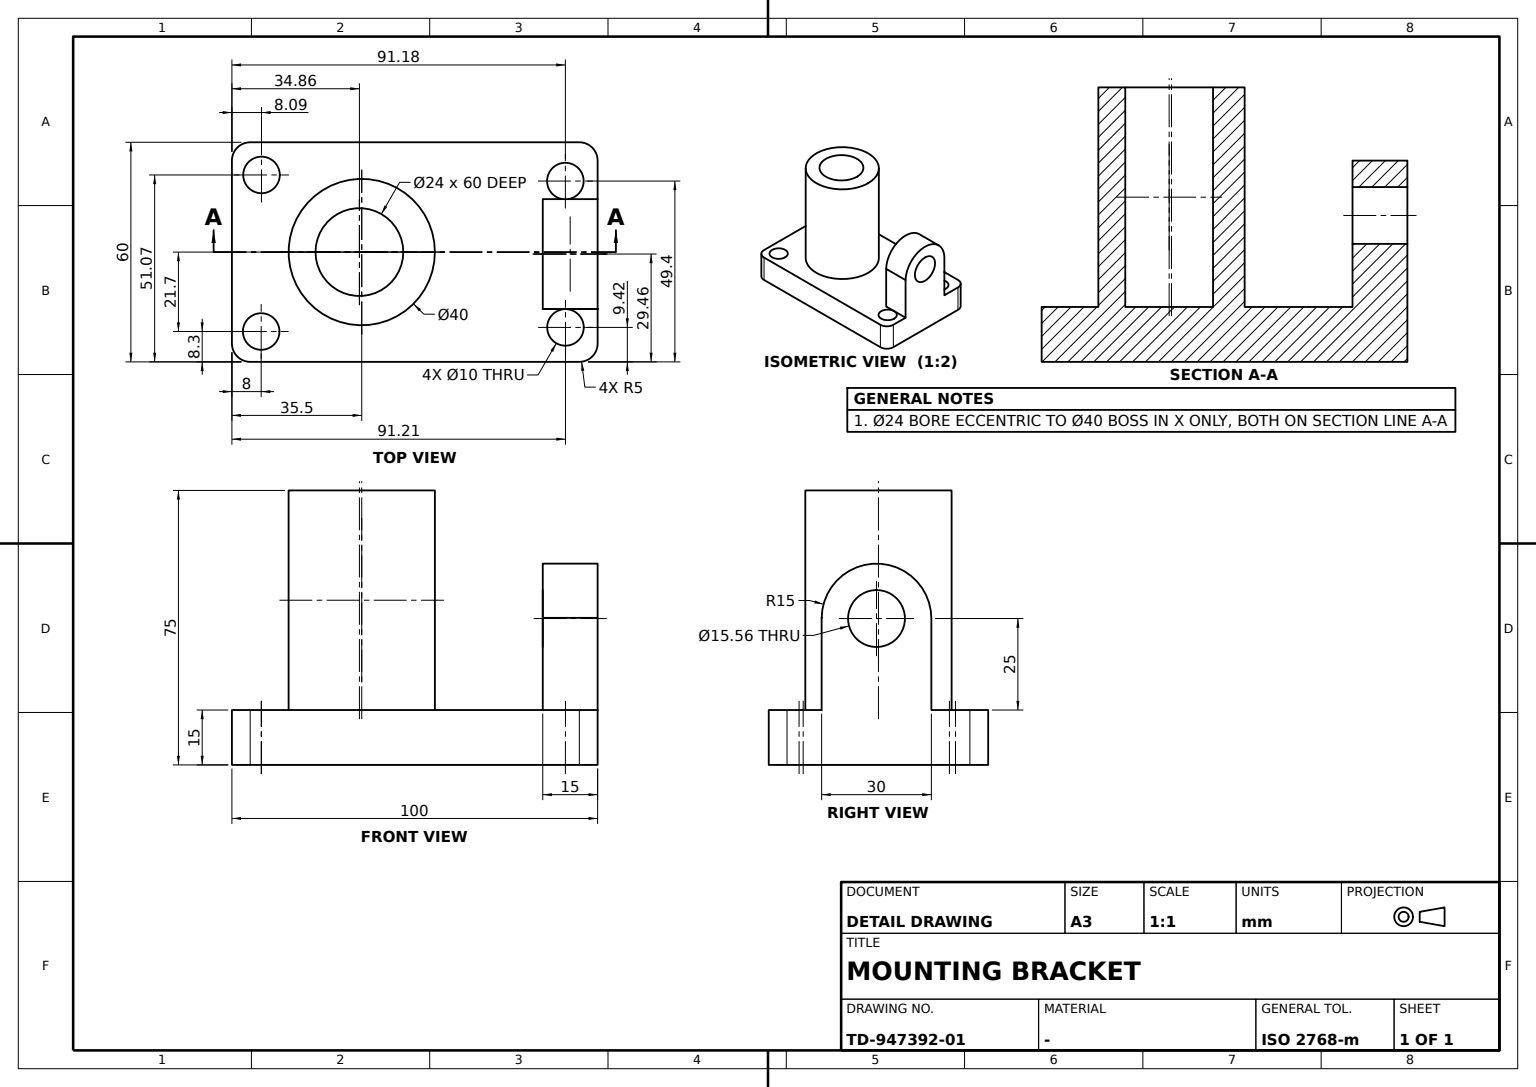
CATIA V5 part; units mm, degrees
sketch "Sketch1" plane through (0, 0, 0) normal (0, 0, 1) x (1, 0, 0)
  point P0 (18.0782, 0)
  line L0 (68.0782, 25) -> (68.0782, -25)
  line L1 (63.0782, -30) -> (-26.9218, -30)
  line L2 (-31.9218, -25) -> (-31.9218, 25)
  line L3 (-26.9218, 30) -> (63.0782, 30)
  point P1 (68.0782, 30)
  point P2 (68.0782, -30)
  point P3 (-31.9218, 30)
  arc A0 (-31.9218, 25) -> (-26.9218, 30) centre (-26.9218, 25) cw
  point P4 (-31.9218, 25)
  point P5 (-26.9218, 30)
  point P6 (-26.9218, 25)
  line L4 (-38.8757, 0) -> (169.5567, 0) construction
  point P7 (-38.8757, 0)
  line L5 (18.0782, -56.7259) -> (18.0782, 81.2462) construction
  point P8 (63.0782, 30)
  point P9 (68.0782, 25)
  arc A1 (68.0782, 25) -> (63.0782, 30) centre (63.0782, 25) ccw
  point P10 (63.0782, -30)
  point P11 (68.0782, -25)
  arc A2 (68.0782, -25) -> (63.0782, -30) centre (63.0782, -25) cw
  point P12 (-26.9218, -30)
  point P13 (-31.9218, -25)
  arc A3 (-31.9218, -25) -> (-26.9218, -30) centre (-26.9218, -25) ccw
  circle A4 centre (-23.8307, 21.07) radius 5
  point P14 (-23.8307, 21.07)
  circle A5 centre (-23.919, -21.7044) radius 5
  circle A6 centre (59.2876, -20.5837) radius 5
  circle A7 centre (59.2609, 19.4027) radius 5
  dimension "distance P3 P1" = 100
  dimension "radius A0" = 5
  dimension "distance P1 P2" = 60
  constraint coincidence P0 x-axis
  constraint coincidence L2 P3
  constraint coincidence L3 P3
  constraint coincidence P7 x-axis
  constraint coincidence P14 A0
  constraint coincidence A4 P6
  constraint vertical L0 y-axis
  constraint vertical L2 y-axis
  constraint vertical L5 y-axis
  constraint horizontal L1 x-axis
  constraint horizontal L3 x-axis
  constraint horizontal L4 x-axis
  constraint equidistance L0 L2 P0
  constraint equidistance L1 L3 P0
  constraint tangency A0 L2
  constraint tangency A0 L3
  constraint symmetry P5 P8 L5
  constraint symmetry P4 P9 L5
  constraint symmetry A0 A1 L5
  constraint symmetry P8 P10 L4
  constraint symmetry P9 P11 L4
  constraint symmetry A1 A2 L4
  constraint symmetry P5 P12 L4
  constraint symmetry P4 P13 L4
  constraint symmetry A0 A3 L4
extrude "Pad1" add sketch "Sketch1" along normal blind 15
sketch "Sketch2" plane through (0, 0, 15) normal (0, 0, 1) x (1, 0, 0)
  circle A0 centre (3.5812, 0) radius 20
  point P0 (3.5812, 0)
  circle A1 centre (2.9417, 0) radius 12
  point P1 (2.9417, 0)
  dimension "radius A0" = 20
  dimension "radius A1" = 12
  constraint coincidence P0 x-axis
  constraint coincidence P1 x-axis
extrude "Pad2" add sketch "Sketch2" along normal blind 60
sketch "Sketch4" plane through (68.0782, 0, 0) normal (1, 0, 0) x (0, 1, 0)
  line L0 (-15.5353, 15) -> (14.4641, 15)
  line L1 (14.4641, 15) -> (14.4641, 40)
  line L2 (-15.5353, 40.1836) -> (-15.5353, 15)
  point P0 (14.4641, 40)
  point P1 (-15.5353, 40.1836)
  line L3 (-25, 15) -> (25, 15) construction
  arc A0 (-15.5353, 40.1836) -> (14.4641, 40) centre (-0.5361, 40) cw
  point P2 (0, 40)
  circle A1 centre (-0.5361, 40) radius 7.7802
  dimension "length L1" = 25
  dimension "distance P0 P1" = 30
  constraint horizontal L0 x-axis
  constraint vertical L1 y-axis
  constraint vertical L2 y-axis
  constraint coincidence L3 L0
  constraint coincidence P2 y-axis
  constraint tangency A0 L1
extrude "Pad3" add sketch "Sketch4" against normal blind 15
sketch "Sketch3" plane through (0, 0, 15) normal (0, 0, 1) x (1, 0, 0)
properties part number "3"
